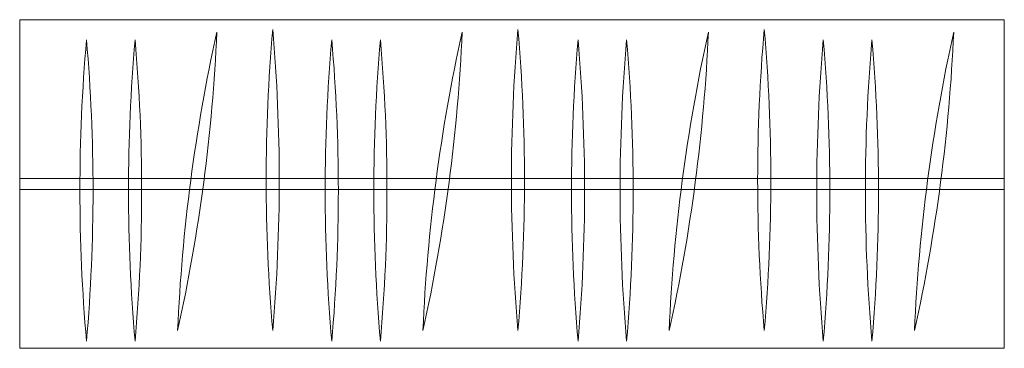
# Model space of a CAD drawing. Units: inches. Extents: x -36302355 to 648, y -221479757 to 75.
# Tile 1 of 37: x -36302355 to -36299747, y -221479757 to -221478888. Entities that reach past the tile are written whole.
import ezdxf

# ---------------------------------------------------------------- set-up
doc = ezdxf.new("R2010")
doc.units = ezdxf.units.IN
doc.header["$MEASUREMENT"] = 0
doc.layers.add('A-FURN-REFR', color=8, linetype='Continuous', lineweight=13)

msp = doc.modelspace()

# ---------------------------------------------------------------- linework, layer by layer
at = {"layer": 'A-FURN-REFR'}
for p, q in [((-36299746.86, -221478887.71), (-36302355.21, -221478887.71)), ((-36302355.21, -221478887.71), (-36302355.21, -221479757.16)), ((-36299746.86, -221478887.71), (-36299746.86, -221479757.16)), ((-36299746.86, -221479307.94), (-36302355.21, -221479307.94)), ((-36299746.86, -221479336.92), (-36302355.21, -221479336.92)), ((-36299746.86, -221479757.16), (-36302355.21, -221479757.16))]:
    msp.add_line(p, q, dxfattribs=at)
for centre, start, end in [((-36306403.36, -221478720.88), 347.50793, 357.50233), ((-36297366.38, -221479909.79), 167.50793, 177.50233), ((-36297127.62, -221479311.76), 175.00282, 184.99718), ((-36306242.47, -221479311.76), 355.00282, 4.99718), ((-36305753.49, -221478720.88), 347.50793, 357.50233), ((-36296716.52, -221479909.79), 167.50793, 177.50233), ((-36296477.76, -221479311.76), 175.00282, 184.99718), ((-36305592.61, -221479311.76), 355.00282, 4.99718), ((-36296064.23, -221479909.79), 167.50793, 177.50233), ((-36305101.21, -221478720.88), 347.50793, 357.50233), ((-36295825.48, -221479311.76), 175.00282, 184.99718), ((-36304940.33, -221479311.76), 355.00282, 4.99718), ((-36295414.37, -221479909.79), 167.50793, 177.50233), ((-36304451.35, -221478720.88), 347.50793, 357.50233), ((-36297620.88, -221479339.81), 175.00282, 184.99718), ((-36306735.73, -221479339.81), 355.00282, 4.99718), ((-36297492.05, -221479339.81), 175.00282, 184.99718), ((-36306606.9, -221479339.81), 355.00282, 4.99718), ((-36296971.02, -221479339.81), 175.00282, 184.99718), ((-36306085.87, -221479339.81), 355.00282, 4.99718), ((-36296842.19, -221479339.81), 175.00282, 184.99718), ((-36305957.04, -221479339.81), 355.00282, 4.99718), ((-36296318.73, -221479339.81), 175.00282, 184.99718), ((-36305433.59, -221479339.81), 355.00282, 4.99718), ((-36296189.9, -221479339.81), 175.00282, 184.99718), ((-36305304.76, -221479339.81), 355.00282, 4.99718), ((-36295668.87, -221479339.81), 175.00282, 184.99718), ((-36304783.72, -221479339.81), 355.00282, 4.99718), ((-36295540.04, -221479339.81), 175.00282, 184.99718), ((-36304654.89, -221479339.81), 355.00282, 4.99718)]:
    msp.add_arc(centre, 4574.81, start, end, dxfattribs=at)

doc.saveas('drawing.dxf')
